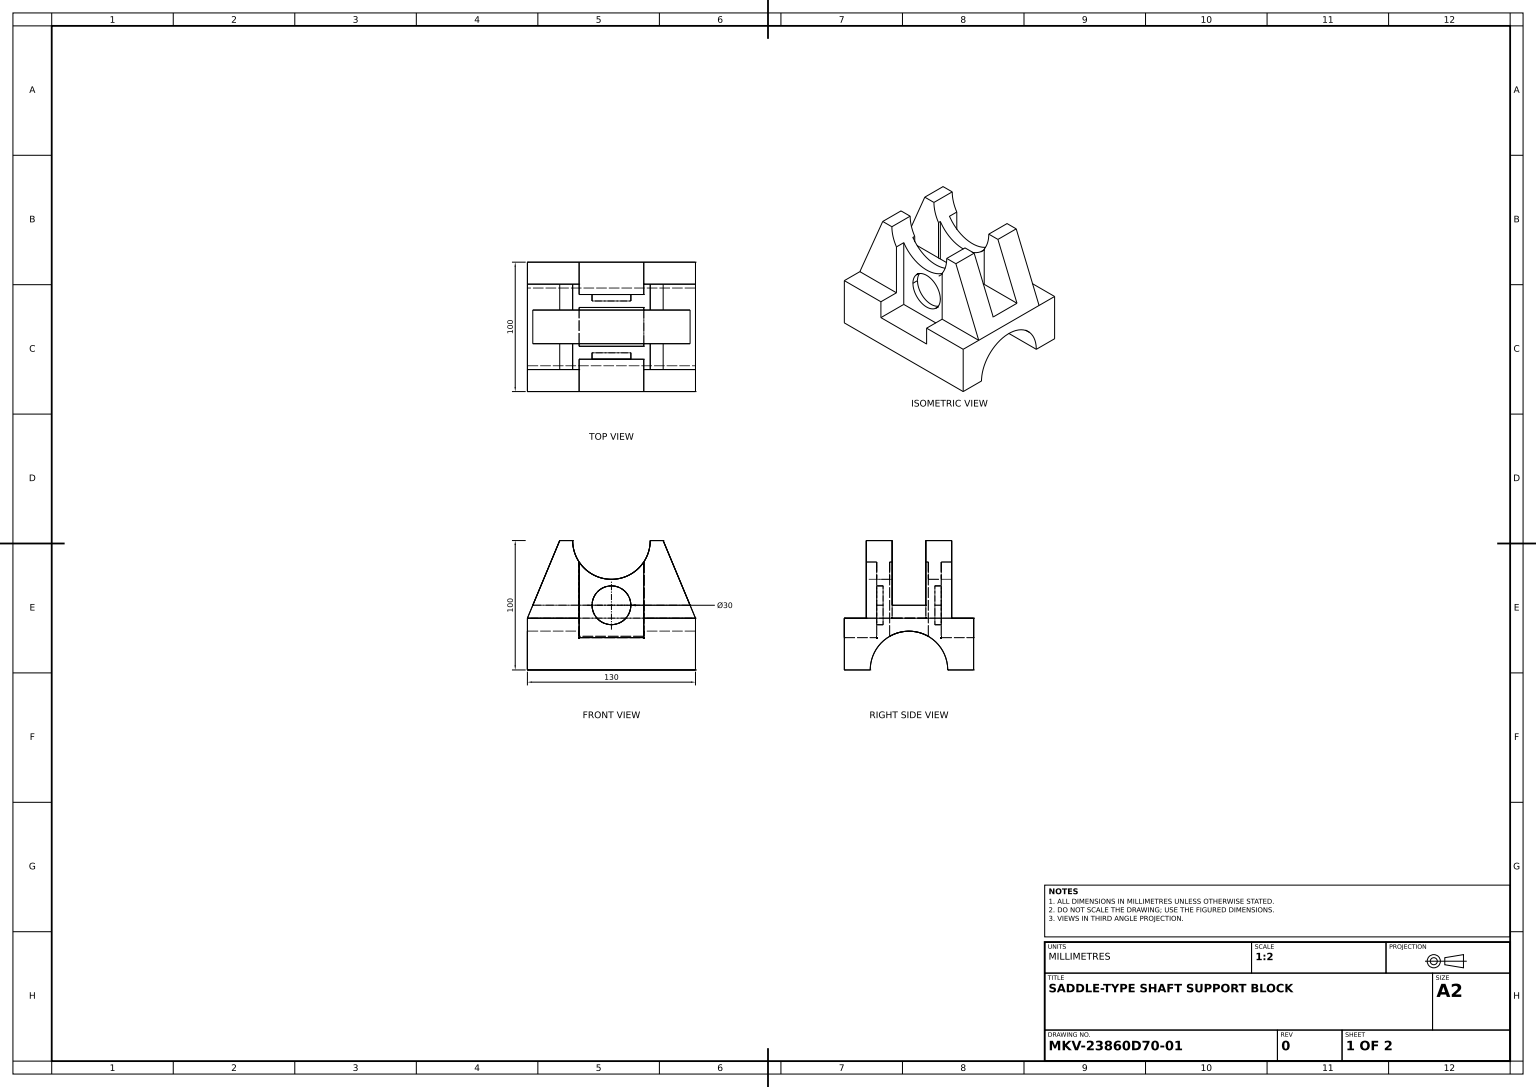
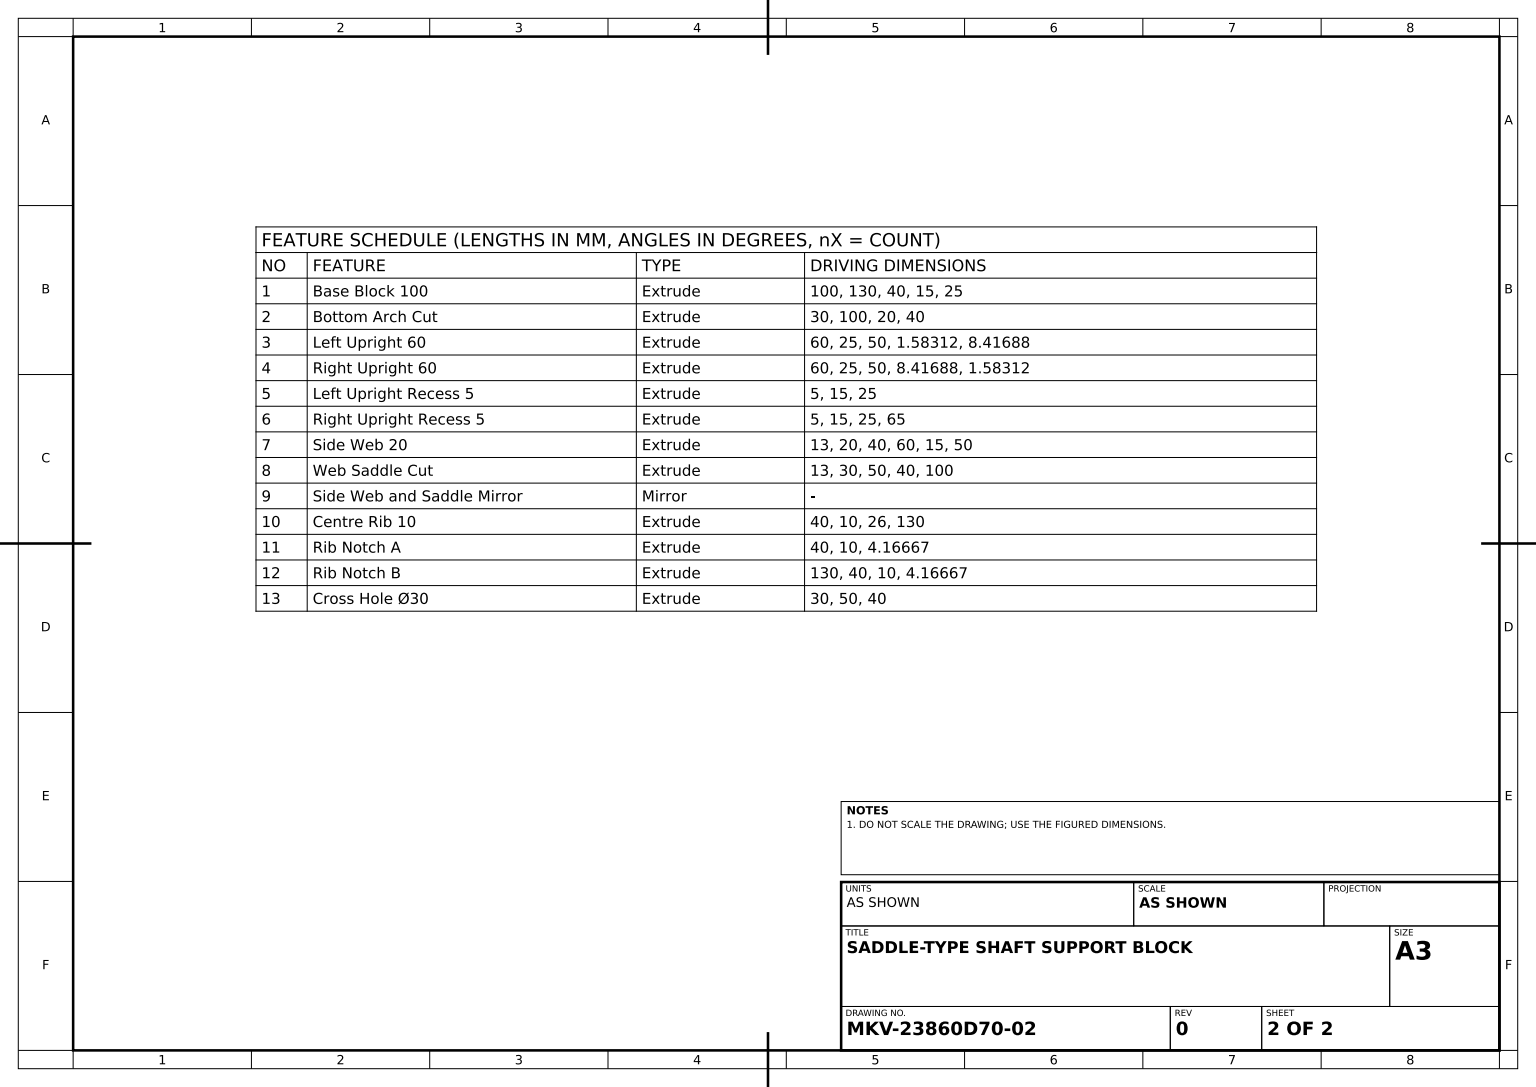
SolidWorks part; units mm, degrees
material "Plain Carbon Steel"
ref_plane "Front Plane" through (0, 0, 0) normal (0, 0, 1) x (1, 0, 0)
ref_plane "Top Plane" through (0, 0, 0) normal (0, 1, 0) x (1, 0, 0)
ref_plane "Right Plane" through (0, 0, 0) normal (1, 0, 0) x (0, 0, -1)
sketch "Base Profile Sketch" plane through (0, 0, 0) normal (0, 0, 1) x (1, 0, 0)
  line L0 (0, 0) -> (130, 0)
  line L1 (130, 0) -> (130, 40)
  line L3 (65, 25) -> (90, 25)
  line L4 (90, 25) -> (40, 25)
  line L5 (40, 25) -> (40, 40)
  line L6 (40, 40) -> (0, 40)
  line L7 (0, 40) -> (0, 0)
  line L8 (130, 40) -> (90, 40)
  line L9 (90, 40) -> (90, 25)
  dimension "D1" = 130
  dimension "D2" = 40
  dimension "D3" = 40
  dimension "D4" = 40
  dimension "D5" = 15
  dimension "D6" = 25
extrude "Base Block 100" add sketch "Base Profile Sketch" along normal mid plane 100 contours L8 L9 L3 L4 L5 L6 L7 L0 L1
sketch "Bottom Arch Sketch" plane through (130, 0, 0) normal (1, 0, 0) x (0, 0, -1)
  line L0 (-50, 0) -> (-30, 0)
  line L1 (50, 0) -> (30, 0)
  line L2 (50, 0) -> (50, 40) construction
  line L3 (-50, 40) -> (50, 40) construction
  circle A1 centre (0, 0) radius 30
  line M4 (-50, 0) -> (50, 0)
  dimension "D1" = 30
  dimension "D2" = 20
  dimension "D3" = 40
  dimension "D5" = 100
extrude "Bottom Arch Cut" cut sketch "Bottom Arch Sketch" against normal through all contours A1 M4
sketch "Left Upright Sketch" plane through (0, 25, 0) normal (0, 1, 0) x (1, 0, 0)
  line L0 (65, -50) -> (65, -25)
  line L1 (65, -25) -> (90, -25)
  line L2 (90, -25) -> (90, -15)
  line L3 (90, -15) -> (40, -15)
  line L4 (40, -15) -> (40, -25)
  line L5 (40, -25) -> (65, -25)
  line L6 (40, -50) -> (40, -16.5831) construction
  line L7 (40, -16.5831) -> (90, -16.5831) construction
  line M1 (90, -16.5831) -> (40, -16.5831)
  line M2 (40, -16.5831) -> (40, -50)
  line M4 (90, -50) -> (90, -16.5831)
  dimension "D1" = 25
  dimension "D2" = 50
  dimension "D3" = 1.5831
  dimension "D4" = 8.4169
extrude "Left Upright 60" add sketch "Left Upright Sketch" along normal blind 60 contours L3 L4 L2 M1 | L5 L1 M2 M4 M1
sketch "Right Upright Sketch" plane through (0, 25, 0) normal (0, 1, 0) x (1, 0, 0)
  line L0 (65, 50) -> (65, 25)
  line L1 (65, 25) -> (90, 25)
  line L2 (90, 25) -> (90, 15)
  line L3 (90, 15) -> (40, 15)
  line L4 (40, 15) -> (40, 25)
  line L5 (40, 25) -> (65, 25)
  line L6 (90, 16.5831) -> (90, 50) construction
  line L7 (90, 16.5831) -> (40, 16.5831) construction
  line M1 (40, 16.5831) -> (90, 16.5831)
  line M2 (90, 16.5831) -> (90, 50)
  line M4 (40, 50) -> (40, 16.5831)
  dimension "D1" = 25
  dimension "D2" = 50
  dimension "D3" = 8.4169
  dimension "D4" = 1.5831
extrude "Right Upright 60" add sketch "Right Upright Sketch" along normal blind 60 contours L5 L1 M4 M1 M2
sketch "Left Upright Recess Sketch" plane through (0, 0, 25) normal (0, 0, 1) x (1, 0, 0)
  line L0 (90, 40) -> (90, 25) construction
  line L1 (40, 25) -> (90, 25) construction
  circle A0 centre (65, 50) radius 15
  dimension "D1" = 15
  dimension "D2" = 25
  dimension "D3" = 25
extrude "Left Upright Recess 5" cut sketch "Left Upright Recess Sketch" against normal blind 5
sketch "Right Upright Recess Sketch" plane through (0, 0, -25) normal (0, 0, -1) x (-1, 0, 0)
  line L0 (-65, 25) -> (-65, 50)
  circle A0 centre (-65, 50) radius 15
  dimension "D1" = 15
  dimension "D2" = 25
  dimension "D3" = 65
  dimension "D4" = 25
extrude "Right Upright Recess 5" cut sketch "Right Upright Recess Sketch" against normal blind 5 contours A0
ref_plane "Side Web Plane 13" through (0, 0, 13) normal (0, 0, 1) x (1, 0, 0)
sketch "Side Web Sketch" plane through (0, 0, 13) normal (0, 0, 1) x (1, 0, 0)
  line L0 (40, 40) -> (40, 100)
  line L1 (25, 100) -> (40, 100)
  line L4 (90, 40) -> (90, 100)
  line L5 (90, 100) -> (105, 100)
  line L6 (130, 40) -> (105, 100)
  line L7 (130, 40) -> (90, 40)
  line L8 (25, 100) -> (0, 40)
  line L9 (0, 40) -> (40, 40)
  dimension "D1" = 40
  dimension "D2" = 40
  dimension "D3" = 60
  dimension "D4" = 15
  dimension "D5" = 50
extrude "Side Web 20" add sketch "Side Web Sketch" along normal blind 20
sketch "Web Saddle Sketch" plane through (0, 0, 13) normal (0, 0, 1) x (1, 0, 0)
  line L0 (40, 100) -> (90, 100)
  circle A0 centre (65, 100) radius 30
  dimension "D1" = 30
  dimension "D2" = 50
  dimension "D3" = 40
  dimension "D4" = 100
extrude "Web Saddle Cut" cut sketch "Web Saddle Sketch" against normal through all both and the other way through all
mirror "Side Web and Saddle Mirror" about plane through (0, 0, 0) normal (0, 0, 1) of "Base Block 100", "Side Web 20", "Web Saddle Cut"
ref_plane "Centre Rib Plane 40" through (0, 40, 0) normal (0, 1, 0) x (1, 0, 0)
sketch "Centre Rib Sketch" plane through (0, 40, 0) normal (0, 1, 0) x (1, 0, 0)
  line L0 (0, 13) -> (0, -13)
  line L1 (0, -13) -> (130, -13)
  line L2 (130, -13) -> (130, 13)
  line L3 (130, 13) -> (0, 13)
  dimension "D1" = 26
  dimension "D2" = 130
extrude "Centre Rib 10" add sketch "Centre Rib Sketch" along normal blind 10
sketch "Rib Notch A Sketch" plane through (0, 0, 13) normal (0, 0, 1) x (1, 0, 0)
  line L0 (4.1667, 50) -> (0, 50)
  line L1 (0, 50) -> (0, 40)
  line L2 (0, 40) -> (4.1667, 50)
  dimension "D1" = 40
  dimension "D2" = 10
  dimension "D3" = 4.1667
extrude "Rib Notch A" cut sketch "Rib Notch A Sketch" against normal through all
sketch "Rib Notch B Sketch" plane through (0, 0, 13) normal (0, 0, 1) x (1, 0, 0)
  line L0 (125.8333, 50) -> (130, 40)
  line L1 (130, 40) -> (130, 50)
  line L2 (130, 50) -> (125.8333, 50)
  dimension "D1" = 130
  dimension "D2" = 40
  dimension "D3" = 10
  dimension "D4" = 4.1667
extrude "Rib Notch B" cut sketch "Rib Notch B Sketch" against normal through all
sketch "Cross Hole Sketch" plane through (130, 0, 0) normal (1, 0, 0) x (0, 0, -1)
  line L1 (-33, 40) -> (33, 40) construction
  circle A0 centre (0, 0) radius 30
  dimension "D1" = 30
  dimension "D2" = 50
  dimension "D3" = 40
extrude "Cross Hole Ø30" cut sketch "Cross Hole Sketch" against normal through all
